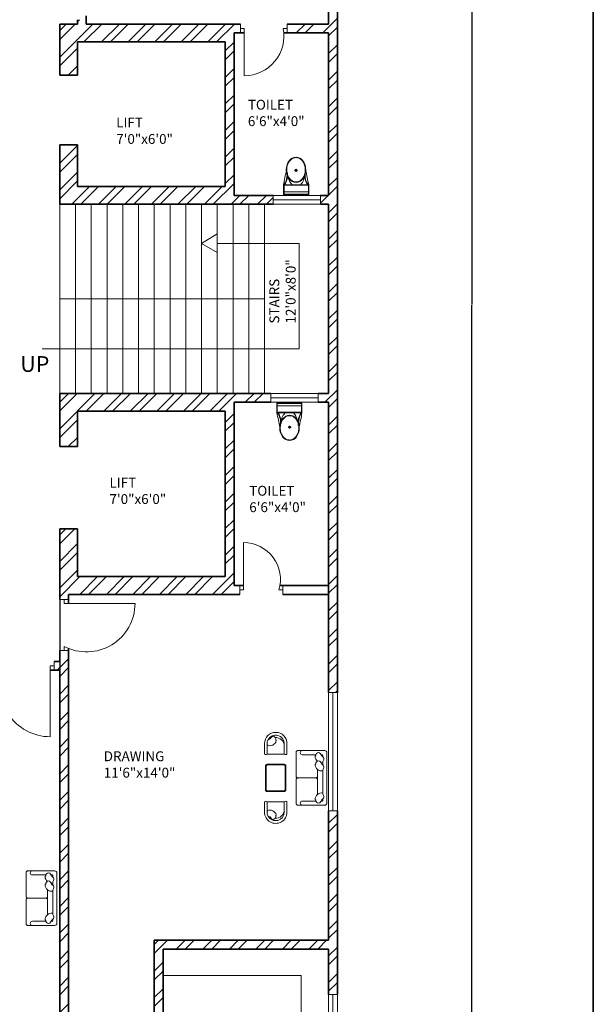
# Model space of a CAD drawing. Units: inches. Extents: x 1885 to 2748, y 783 to 2421.
# Tile 54 of 117: x 2457 to 2748, y 1350 to 1850. Entities that reach past the tile are written whole.
import ezdxf

# ---------------------------------------------------------------- set-up
doc = ezdxf.new("R2010")
doc.units = ezdxf.units.IN
for name, color, linetype, lineweight in [('A-ANNO-DIMS', 2, 'Continuous', 18), ('A-ANNO-SYMB', 81, 'Continuous', 18), ('A-ANNO-TTLB', 7, 'Continuous', 35), ('A-AREA-IDEN', 7, 'Continuous', 18), ('A-DOOR', 31, 'Continuous', 18), ('A-FLOR-CASE', 9, 'Continuous', 18), ('A-FLOR-FIXT', 8, 'Continuous', 18), ('A-FLOR-STRS', 81, 'Continuous', 18), ('A-FURN', 8, 'Continuous', 13), ('A-GLAZ', 181, 'Continuous', 18), ('A-WALL', 7, 'Continuous', 35)]:
    doc.layers.add(name, color=color, linetype=linetype, lineweight=lineweight)
doc.layers.add('A-WALL-PATT', color=85, linetype='Continuous', lineweight=13, true_color=0x58ba48)
doc.styles.get("Standard").update_dxf_attribs({"font": 'arial.ttf'})
doc.dimstyles.get("Standard").update_dxf_attribs({"dimtxt": 0.18, "dimasz": 0.18, "dimexe": 0.18, "dimexo": 0.0625, "dimgap": 0.09, "dimtad": 0, "dimtih": 1, "dimtoh": 1, "dimdec": 4, "dimzin": 0, "dimdsep": 46, "dimtxsty": 'Standard', "dimcen": 0.09, "dimadec": 0, "dimazin": 0, "dimtfac": 1, "dimtdec": 4, "dimtofl": 0, "dimtmove": 0, "dimatfit": 3, "dimfxl": 1, "dimtolj": 1, "dimtzin": 0, "dimarcsym": 0})

# ---------------------------------------------------------------- blocks, each defined once
blk = doc.blocks.new('A$C31115884')
for p, q in [((283, 498), (223, 498)), ((258, 466), (258, 523)), ((0, 200), (0, 0)), ((520, 200), (0, 200)), ((510, 54), (0, 54)), ((10, 190), (10, 10)), ((510, 190), (10, 190)), ((10, 10), (510, 10)), ((510, 10), (510, 190)), ((520, 0), (520, 200)), ((0, 0), (520, 0))]:
    blk.add_line(p, q)
blk.add_circle((256, 496), 23.6)
for centre, radius, start, end in [((2778, -205), 2807, 165.4549, 171.7133), ((-295, 403), 365, 324.2091, 9.3499), ((-295, 403), 375, 324.2091, 9.3499), ((139, 406), 293, 315.8436, 2.6563), ((806, 403), 375, 179.2036, 215.7909), ((806, 403), 365, 170.6501, 215.7909), ((3237, 905), 2807, 188.2867, 194.5451), ((384, 406), 293, 190.2774, 224.1564)]:
    blk.add_arc(centre, radius, start, end)
blk.add_ellipse((256, 510), major_axis=(0, -261), ratio=0.772727)
blk.add_open_spline([(256, 259), (263, 259), (270, 260), (288, 262), (299, 265), (320, 273), (330, 278), (350, 291), (360, 299), (378, 316), (386, 326), (402, 347), (409, 358), (421, 383), (427, 395), (436, 422), (440, 436), (445, 465), (447, 480), (448, 509), (448, 524), (445, 553), (443, 568), (436, 596), (432, 610), (422, 636), (416, 649), (402, 672), (395, 683), (379, 703), (370, 712), (351, 728), (341, 735), (321, 746), (310, 751), (289, 757), (278, 759), (256, 761), (245, 761), (223, 757), (212, 754), (191, 746), (181, 741), (161, 728), (151, 720), (133, 703), (125, 693), (110, 672), (103, 660), (90, 636), (85, 623), (76, 596), (72, 582), (67, 553), (66, 538), (64, 509), (65, 494), (68, 465), (70, 450), (77, 422), (81, 408), (91, 382), (97, 370), (111, 346), (118, 335), (135, 316), (144, 307), (162, 291), (172, 284), (193, 273), (203, 269), (225, 262), (236, 260), (250, 259), (253, 259), (256, 259)], degree=3, knots=[0, 0, 0, 0, 0.110105, 0.110105, 0.285049, 0.285049, 0.459994, 0.459994, 0.634938, 0.634938, 0.809882, 0.809882, 0.984827, 0.984827, 1.159771, 1.159771, 1.334715, 1.334715, 1.50966, 1.50966, 1.684604, 1.684604, 1.859549, 1.859549, 2.034493, 2.034493, 2.209437, 2.209437, 2.384382, 2.384382, 2.559326, 2.559326, 2.73427, 2.73427, 2.909215, 2.909215, 3.084159, 3.084159, 3.259103, 3.259103, 3.434048, 3.434048, 3.608992, 3.608992, 3.783936, 3.783936, 3.958881, 3.958881, 4.133825, 4.133825, 4.30877, 4.30877, 4.483714, 4.483714, 4.658658, 4.658658, 4.833603, 4.833603, 5.008547, 5.008547, 5.183491, 5.183491, 5.358436, 5.358436, 5.53338, 5.53338, 5.708324, 5.708324, 5.883269, 5.883269, 6.058213, 6.058213, 6.233158, 6.233158, 6.283185, 6.283185, 6.283185, 6.283185])
blk = doc.blocks.new('A$C1352')
at = {"color": 0}
for points in [[(0.003, 0.053), (0.003, 0.553, -0.414214), (0.053, 0.603), (0.753, 0.603, -0.414214), (0.803, 0.553), (0.803, 0.053, -0.414214), (0.753, 0.003), (0.053, 0.003, -0.414214)], [(0.023, 0.053), (0.023, 0.553, -0.414214), (0.053, 0.583), (0.753, 0.583, -0.414214), (0.783, 0.553), (0.783, 0.053, -0.414214), (0.753, 0.023), (0.053, 0.023, -0.414214)]]:
    blk.add_lwpolyline(points, format="xyb", close=True, dxfattribs=at)
blk = doc.blocks.new('CHAIR-LOUNGE')
blk.add_line((1.39, 5.7), (1.38, 10.98))
at = {"ltscale": 0.03}
blk.add_lwpolyline([(1.38, 10.98, 0.369229), (0, 10.98), (0, 5.7, 1), (11.42, 5.71), (11.42, 10.99, 0.369229), (10.03, 10.99)], format="xyb", close=True, dxfattribs=at)
blk.add_lwpolyline([(1.88, 3.71, 0.785087), (10.04, 5.71), (10.03, 10.99)], format="xyb")
for centre, radius, start, end in [((3.01, 5.02), 1.73, 145.8599, 267.0078), ((5.71, 5.71), 4.33, 180.0539, 181.1464), ((2.75, 3.42), 3.35, 15.7143, 112.9857), ((5.71, 6.93), 4.33, 266.342, 0.0539), ((4.77, 3.91), 1.95, 198.6466, 265.0001), ((3.98, 3.63), 1.78, 290.5305, 13.3597), ((5.79, 4.23), 0.207, 246.2577, 29.3762)]:
    blk.add_arc(centre, radius, start, end)
blk = doc.blocks.new('WIN-24')
for p, q in [((0, 4.5), (0, 0)), ((0, 4.5), (24, 4.5)), ((0, 0), (0, 2.25)), ((0, 2.25), (24, 2.25)), ((24, 2.25), (24, 4.5)), ((24, 4.5), (24, 0)), ((24, 0), (0, 0))]:
    blk.add_line(p, q)
blk = doc.blocks.new('WIN-36')
for p, q in [((0, 36), (4.5, 36)), ((0, 36), (0, 0)), ((4.5, 36), (2.25, 36)), ((2.25, 36), (2.25, 0)), ((4.5, 36), (4.5, 0)), ((2.25, 0), (0, 0)), ((0, 0), (4.5, 0))]:
    blk.add_line(p, q)
blk = doc.blocks.new('WIN-60-ALT')
for p, q in [((0, 60), (4.5, 60)), ((0, 60), (0, 0)), ((4.5, 60), (2.25, 60)), ((2.25, 60), (2.25, 0)), ((4.5, 0), (4.5, 60)), ((4.5, 0), (0, 0)), ((2.25, 0), (4.5, 0))]:
    blk.add_line(p, q)
blk = doc.blocks.new('*D44')
at = {"layer": 'A-ANNO-DIMS', "color": 0, "lineweight": -2, "transparency": 16777216}
for p, q in [((2618.34, 2352.51), (2686.7, 2352.51)), ((2686.52, 2352.33), (2686.52, 1705.19)), ((2686.52, 1057.69), (2686.52, 1704.82)), ((2618.34, 1057.51), (2686.7, 1057.51))]:
    blk.add_line(p, q, dxfattribs=at)
at = {"layer": 'A-ANNO-DIMS', "color": 0, "transparency": 16777216}
for points in [[(2686.49, 2352.33), (2686.55, 2352.33), (2686.52, 2352.51)], [(2686.49, 1057.69), (2686.55, 1057.69), (2686.52, 1057.51)]]:
    blk.add_solid(points, dxfattribs=at)
at = {"layer": 'Defpoints', "color": 0, "transparency": 16777216}
for p in [(2618.27, 2352.51), (2686.52, 2352.51), (2618.27, 1057.51)]:
    blk.add_point(p, dxfattribs=at)
at = {"layer": 'A-ANNO-DIMS', "color": 0, "transparency": 16777216, "insert": (2686.52, 1705.01), "char_height": 0.18, "attachment_point": 5}
blk.add_mtext('\\A1;1295', dxfattribs=at)
blk = doc.blocks.new('*D55')
at = {"layer": 'A-ANNO-DIMS', "color": 0, "lineweight": -2, "transparency": 16777216}
for p, q in [((2447.27, 1557.94), (2447.27, 922.48)), ((2477.27, 1557.94), (2477.27, 922.48)), ((2447.45, 922.66), (2462.06, 922.66)), ((2477.09, 922.66), (2462.49, 922.66))]:
    blk.add_line(p, q, dxfattribs=at)
at = {"layer": 'A-ANNO-DIMS', "color": 0, "transparency": 16777216}
for points in [[(2447.45, 922.69), (2447.45, 922.63), (2447.27, 922.66)], [(2477.09, 922.69), (2477.09, 922.63), (2477.27, 922.66)]]:
    blk.add_solid(points, dxfattribs=at)
at = {"layer": 'Defpoints', "color": 0, "transparency": 16777216}
for p in [(2447.27, 1558.01), (2477.27, 1558.01), (2477.27, 922.66)]:
    blk.add_point(p, dxfattribs=at)
at = {"layer": 'A-ANNO-DIMS', "color": 0, "transparency": 16777216, "insert": (2462.27, 922.66), "char_height": 0.18, "attachment_point": 5}
blk.add_mtext('\\A1;30', dxfattribs=at)

msp = doc.modelspace()

# ---------------------------------------------------------------- hatches: boundary and pattern name
at = {"layer": 'A-WALL-PATT'}
h = msp.add_hatch(dxfattribs=at)
h.set_pattern_fill('ANSI32', color=256)
h.paths.add_polyline_path([(2007.77, 2318.01), (1980.77, 2318.01), (1980.77, 2281.22), (1985.27, 2281.22), (1985.27, 2313.51), (2007.77, 2313.51), (2007.77, 2315.76)])
h.paths.add_polyline_path([(2094.32, 2318.01), (2067.77, 2318.01), (2067.77, 2313.51), (2094.32, 2313.51), (2094.32, 2315.76)])
h.paths.add_polyline_path([(2131.37, 2315.76), (2131.37, 2318.01), (2131.19, 2318.01), (2112.61, 2318.01), (2112.61, 2313.51), (2117.27, 2313.51), (2117.27, 2255.2), (2121.77, 2255.2), (2121.77, 2313.51), (2131.37, 2313.51)])
h.paths.add_polyline_path([(2190.51, 2318.01), (2155.37, 2318.01), (2155.37, 2313.51), (2169.77, 2313.51), (2169.77, 2229.51), (2121.77, 2229.51), (2121.77, 2233.45), (2119.52, 2233.45), (2117.27, 2233.45), (2117.27, 2201.1), (2121.77, 2201.1), (2121.77, 2225.01), (2169.77, 2225.01), (2169.77, 2165.01), (2306.27, 2165.01), (2306.27, 2066.01), (2310.77, 2066.01), (2344.27, 2066.01), (2486.27, 2066.01), (2486.27, 1886.01), (2483.02, 1886.01), (2483.02, 1881.51), (2486.27, 1881.51), (2486.27, 1880.68), (2490.77, 1880.68), (2490.77, 2070.51), (2344.27, 2070.51), (2310.77, 2070.51), (2310.77, 2165.01), (2310.77, 2173.64), (2308.52, 2173.64), (2306.27, 2173.64), (2306.27, 2169.51), (2174.27, 2169.51), (2174.27, 2313.51), (2190.51, 2313.51), (2190.51, 2315.76)])
h.paths.add_polyline_path([(1985.27, 2221.22), (1980.77, 2221.22), (1980.77, 2165.01), (1992.77, 2165.01), (1992.77, 2141.93), (1997.27, 2141.93), (1997.27, 2165.01), (2117.27, 2165.01), (2117.27, 2163.13), (2121.77, 2163.13), (2121.77, 2172.73), (2119.52, 2172.73), (2117.27, 2172.73), (2117.27, 2169.51), (1985.27, 2169.51)])
h.paths.add_polyline_path([(1997.27, 2105.93), (1992.77, 2105.93), (1992.77, 2070.51), (2016.77, 2070.51), (2016.77, 2059.12), (2019.02, 2059.12), (2021.27, 2059.12), (2021.27, 2070.51), (2117.27, 2070.51), (2117.27, 2022.51), (2114.42, 2022.51), (2114.42, 2018.01), (2123.63, 2018.01), (2123.63, 2020.26), (2123.63, 2022.51), (2121.77, 2022.51), (2121.77, 2142.59), (2119.52, 2142.59), (2117.27, 2142.59), (2117.27, 2075.01), (1997.27, 2075.01)])
h.paths.add_polyline_path([(2092.03, 2020.26), (2092.03, 2022.51), (2021.27, 2022.51), (2021.27, 2035.12), (2016.77, 2035.12), (2016.77, 2018.01), (2016.77, 1978.78), (2021.27, 1978.78), (2021.27, 2018.01), (2092.03, 2018.01)])
h.paths.add_polyline_path([(2260.94, 2022.51), (2153.1, 2022.51), (2153.1, 2020.26), (2153.1, 2018.01), (2155.27, 2018.01), (2155.27, 1886.01), (2107.63, 1886.01), (2107.63, 1881.51), (2182.91, 1881.51), (2182.91, 1883.76), (2182.91, 1886.01), (2159.77, 1886.01), (2159.77, 2018.01), (2260.94, 2018.01), (2260.94, 2020.26)])
h.paths.add_polyline_path([(2047.63, 1883.76), (2047.63, 1886.01), (2021.27, 1886.01), (2021.27, 1918.78), (2019.02, 1918.78), (2016.77, 1918.78), (2016.77, 1881.51), (2047.63, 1881.51)])
h.paths.add_polyline_path([(2306.36, 1883.76), (2306.36, 1886.01), (2296.27, 1886.01), (2296.27, 1982.01), (2316.54, 1982.01), (2316.54, 1984.26), (2316.54, 1986.51), (2296.27, 1986.51), (2296.27, 2022.51), (2289.28, 2022.51), (2289.28, 2018.01), (2291.77, 2018.01), (2291.77, 1886.01), (2242.91, 1886.01), (2242.91, 1881.51), (2306.36, 1881.51)], flags=17)
h.paths.add_polyline_path([(1985.27, 1843.01), (2021.6, 1843.01), (2021.53, 1845.44), (2021.48, 1847.51), (1980.77, 1847.51), (1980.77, 1809.45), (1985.27, 1809.45)])
h.paths.add_polyline_path([(2131.48, 1845.26), (2131.48, 1847.51), (2081.53, 1847.51), (2081.53, 1843.01), (2117.27, 1843.01), (2117.27, 1784.15), (2119.52, 1784.15), (2121.77, 1784.15), (2121.77, 1843.01), (2131.48, 1843.01)])
h.paths.add_polyline_path([(2203.89, 1847.51), (2155.48, 1847.51), (2155.48, 1843.01), (2169.77, 1843.01), (2169.77, 1759.01), (2121.77, 1759.01), (2121.77, 1761.46), (2117.27, 1761.46), (2117.27, 1730.43), (2121.77, 1730.43), (2121.77, 1754.51), (2177.42, 1754.51), (2177.42, 1756.76), (2177.42, 1759.01), (2174.27, 1759.01), (2174.27, 1843.01), (2203.89, 1843.01)])
h.paths.add_polyline_path([(2335.55, 1845.26), (2335.55, 1847.51), (2239.89, 1847.51), (2239.89, 1843.01), (2306.27, 1843.01), (2306.27, 1759.01), (2199.49, 1759.01), (2199.49, 1754.51), (2310.77, 1754.51), (2310.77, 1843.01), (2335.55, 1843.01)])
h.paths.add_polyline_path([(2348.77, 2022.51), (2344.27, 2022.51), (2344.27, 1986.51), (2341.68, 1986.51), (2341.68, 1982.01), (2344.27, 1982.01), (2344.27, 1886.01), (2330.36, 1886.01), (2330.36, 1881.51), (2361.63, 1881.51), (2361.63, 1883.76), (2361.63, 1886.01), (2348.77, 1886.01)], flags=17)
h.paths.add_polyline_path([(2283.25, 2315.76), (2283.25, 2318.01), (2238.51, 2318.01), (2238.51, 2313.51), (2283.25, 2313.51)], flags=17)
h.paths.add_polyline_path([(2363.27, 2348.01), (2388.68, 2348.01), (2388.68, 2350.26), (2388.68, 2352.51), (2358.77, 2352.51), (2358.77, 2348.01), (2358.77, 2318.01), (2344.48, 2318.01), (2344.48, 2313.51), (2358.77, 2313.51), (2358.77, 2229.51), (2310.77, 2229.51), (2310.77, 2231.95), (2306.27, 2231.95), (2306.27, 2205.61), (2310.77, 2205.61), (2310.77, 2225.01), (2358.77, 2225.01), (2358.77, 2211.51), (2452.33, 2211.51), (2452.33, 2213.76), (2452.33, 2216.01), (2363.27, 2216.01), (2363.27, 2318.01)])
h.paths.add_polyline_path([(2310.77, 2313.51), (2320.48, 2313.51), (2320.48, 2315.76), (2320.48, 2318.01), (2302.73, 2318.01), (2302.73, 2313.51), (2306.27, 2313.51), (2306.27, 2251.08), (2310.77, 2251.08)], flags=17)
h.paths.add_polyline_path([(2490.77, 2352.51), (2486.27, 2352.51), (2448.68, 2352.51), (2448.68, 2348.01), (2486.27, 2348.01), (2486.27, 2318.01), (2486.27, 2216.01), (2481.78, 2216.01), (2481.78, 2211.51), (2486.27, 2211.51), (2486.27, 2165.01), (2493.29, 2165.01), (2493.29, 2167.26), (2493.29, 2169.51), (2490.77, 2169.51), (2490.77, 2313.51), (2494.43, 2313.51), (2494.43, 2318.01), (2490.77, 2318.01)])
h.paths.add_polyline_path([(2534.65, 2318.01), (2515.69, 2318.01), (2515.69, 2313.51), (2534.65, 2313.51), (2534.65, 2315.76)])
h.paths.add_polyline_path([(2618.27, 2318.01), (2594.65, 2318.01), (2594.65, 2313.51), (2613.77, 2313.51), (2613.77, 2281.71), (2618.27, 2281.71)])
h.paths.add_polyline_path([(2618.27, 2221.71), (2613.77, 2221.71), (2613.77, 2169.51), (2554.02, 2169.51), (2554.02, 2165.01), (2613.77, 2165.01), (2613.77, 2152.88), (2618.27, 2152.88)])
h.paths.add_polyline_path([(2618.27, 2128.88), (2616.02, 2128.88), (2613.77, 2128.88), (2613.77, 2117.01), (2529.77, 2117.01), (2529.77, 2165.01), (2532.85, 2165.01), (2532.85, 2169.51), (2522.87, 2169.51), (2522.87, 2165.01), (2525.27, 2165.01), (2525.27, 2117.01), (2525.27, 2112.51), (2525.27, 2108.58), (2529.77, 2108.58), (2529.77, 2112.51), (2613.77, 2112.51), (2613.77, 2080.19), (2618.27, 2080.19)])
h.paths.add_polyline_path([(2618.27, 2044.19), (2616.02, 2044.19), (2613.77, 2044.19), (2613.77, 2015.51), (2529.77, 2015.51), (2529.77, 2088.58), (2527.52, 2088.58), (2525.27, 2088.58), (2525.27, 2011.01), (2613.77, 2011.01), (2613.77, 1956.75), (2618.27, 1956.75)])
h.paths.add_polyline_path([(2618.27, 1881.51), (2618.27, 1896.75), (2613.77, 1896.75), (2613.77, 1881.51), (2613.77, 1847.51), (2592.71, 1847.51), (2592.71, 1843.01), (2613.77, 1843.01), (2613.77, 1765.01), (2613.77, 1760.51), (2609.62, 1760.51), (2609.62, 1756.01), (2613.77, 1756.01), (2613.77, 1660.01), (2608.54, 1660.01), (2608.54, 1655.51), (2613.77, 1655.51), (2613.77, 1508.16), (2618.27, 1508.16)])
h.paths.add_polyline_path([(2565.77, 1843.01), (2569, 1843.01), (2569, 1847.51), (2490.77, 1847.51), (2490.77, 1849.7), (2488.52, 1849.7), (2486.27, 1849.7), (2486.27, 1847.51), (2477.27, 1847.51), (2477.27, 1838.51), (2477.27, 1821.49), (2486.27, 1821.49), (2486.27, 1838.51), (2561.27, 1838.51), (2561.27, 1765.01), (2486.27, 1765.01), (2486.27, 1786.16), (2477.27, 1786.16), (2477.27, 1765.01), (2477.27, 1756.01), (2486.27, 1756.01), (2565.77, 1756.01), (2585.62, 1756.01), (2585.62, 1758.26), (2585.62, 1760.51), (2565.77, 1760.51), (2565.77, 1765.01)])
h.paths.add_polyline_path([(2486.27, 1651.01), (2561.27, 1651.01), (2561.27, 1567.01), (2486.27, 1567.01), (2486.27, 1591.32), (2477.27, 1591.32), (2477.27, 1567.01), (2477.27, 1558.01), (2477.27, 1555.44), (2481.77, 1555.44), (2481.77, 1558.01), (2568.65, 1558.01), (2568.65, 1560.26), (2568.65, 1562.51), (2565.77, 1562.51), (2565.77, 1655.51), (2584.54, 1655.51), (2584.54, 1657.76), (2584.54, 1660.01), (2565.77, 1660.01), (2486.27, 1660.01), (2477.27, 1660.01), (2477.27, 1651.01), (2477.27, 1632.99), (2486.27, 1632.99)])
h.paths.add_polyline_path([(2449.97, 1883.76), (2449.97, 1886.01), (2421.63, 1886.01), (2421.63, 1881.51), (2449.97, 1881.51)], flags=17)
h.paths.add_polyline_path([(2447.27, 1847.51), (2395.55, 1847.51), (2395.55, 1843.01), (2442.77, 1843.01), (2442.77, 1809.27), (2447.27, 1809.27)])
h.paths.add_polyline_path([(1985.27, 1749.45), (1980.77, 1749.45), (1980.77, 1694.5), (1985.27, 1694.5), (1985.27, 1694.51), (1986.9, 1694.51), (1986.9, 1697.78), (1986.9, 1699.01), (1985.27, 1699.01)])
h.paths.add_polyline_path([(2152.77, 1699.01), (2121.77, 1699.01), (2121.77, 1703.67), (2119.52, 1703.67), (2117.27, 1703.67), (2117.27, 1699.01), (2009.22, 1699.01), (2009.22, 1694.51), (2148.27, 1694.51), (2148.27, 1692.63), (2152.77, 1692.63)])
h.paths.add_polyline_path([(2016.27, 1694.51), (2011.77, 1694.51), (2011.77, 1558.01), (2040.81, 1558.01), (2040.81, 1560.26), (2040.81, 1562.51), (2016.27, 1562.51)])
h.paths.add_polyline_path([(2152.77, 1663.02), (2150.52, 1663.02), (2148.27, 1663.02), (2148.27, 1562.51), (2100.81, 1562.51), (2100.81, 1558.01), (2165.12, 1558.01), (2165.12, 1560.26), (2165.12, 1562.51), (2152.77, 1562.51), (2152.77, 1610.51), (2224.77, 1610.51), (2224.77, 1607.99), (2229.27, 1607.99), (2229.27, 1615.01), (2152.77, 1615.01)])
h.paths.add_polyline_path([(2238.61, 1560.26), (2238.61, 1562.51), (2229.27, 1562.51), (2229.27, 1588.76), (2227.02, 1588.76), (2224.77, 1588.77), (2224.77, 1562.51), (2189.12, 1562.51), (2189.12, 1558.01), (2238.61, 1558.01)])
h.paths.add_polyline_path([(2336.02, 1560.26), (2336.02, 1562.51), (2310.77, 1562.51), (2310.77, 1656.35), (2308.52, 1656.35), (2306.27, 1656.35), (2306.27, 1562.51), (2286.61, 1562.51), (2286.61, 1558.01), (2336.02, 1558.01)])
h.paths.add_polyline_path([(2447.27, 1690.97), (2445.02, 1690.97), (2442.77, 1690.97), (2442.77, 1687.01), (2306.27, 1687.01), (2306.27, 1680.75), (2310.77, 1680.75), (2310.77, 1682.51), (2442.77, 1682.51), (2442.77, 1562.51), (2396.02, 1562.51), (2396.02, 1558.01), (2447.27, 1558.01)])
h.paths.add_polyline_path([(2447.27, 1749.27), (2445.02, 1749.27), (2442.77, 1749.27), (2442.77, 1717.23), (2447.27, 1717.23)])
h.paths.add_polyline_path([(2044.67, 1521.76), (2044.67, 1524.01), (2007.27, 1524.01), (2007.27, 1503.49), (2009.52, 1503.49), (2011.77, 1503.49), (2011.77, 1519.51), (2044.67, 1519.51)])
h.paths.add_polyline_path([(2177.97, 1521.76), (2177.97, 1524.01), (2104.67, 1524.01), (2104.67, 1519.51), (2145.77, 1519.51), (2145.77, 1387.51), (2143.37, 1387.51), (2143.37, 1383.01), (2251.59, 1383.01), (2251.59, 1385.26), (2251.59, 1387.51), (2150.27, 1387.51), (2150.27, 1519.51), (2177.97, 1519.51)])
h.paths.add_polyline_path([(2298.7, 1524.01), (2237.97, 1524.01), (2237.97, 1519.51), (2282.27, 1519.51), (2282.27, 1387.51), (2279.68, 1387.51), (2279.68, 1383.01), (2286.77, 1383.01), (2286.77, 1419.01), (2312.45, 1419.01), (2312.45, 1421.26), (2312.45, 1423.51), (2286.77, 1423.51), (2286.77, 1519.51), (2298.7, 1519.51), (2298.7, 1521.72)], flags=17)
h.paths.add_polyline_path([(2361.9, 1521.76), (2361.9, 1524.01), (2322.7, 1524.01), (2322.7, 1519.51), (2334.77, 1519.51), (2334.77, 1423.51), (2331.93, 1423.51), (2331.93, 1419.01), (2334.77, 1419.01), (2334.77, 1387.51), (2334.77, 1383.23), (2339.27, 1383.23), (2339.27, 1387.51), (2339.27, 1519.51), (2361.9, 1519.51)], flags=17)
h.paths.add_polyline_path([(2447.27, 1521.76), (2447.27, 1524.01), (2421.9, 1524.01), (2421.9, 1519.51), (2447.27, 1519.51)], flags=17)
h.paths.add_polyline_path([(2481.77, 1529.6), (2479.52, 1529.6), (2477.27, 1529.6), (2477.27, 1524.01), (2474.49, 1524.01), (2474.49, 1519.51), (2477.27, 1519.51), (2477.27, 1334.51), (2296.77, 1334.51), (2296.77, 1240.51), (2160.27, 1240.51), (2160.27, 1180.51), (2112.27, 1180.51), (2112.27, 1207.69), (2110.02, 1207.69), (2107.77, 1207.69), (2107.77, 1171.61), (2112.27, 1171.61), (2112.27, 1176.01), (2160.27, 1176.01), (2160.27, 1092.01), (2144.22, 1092.01), (2144.22, 1087.51), (2189.5, 1087.51), (2189.5, 1089.76), (2189.5, 1092.01), (2164.77, 1092.01), (2164.77, 1236.01), (2296.77, 1236.01), (2296.77, 1231.91), (2301.27, 1231.91), (2301.27, 1330.01), (2481.77, 1330.01), (2481.77, 1387.51)])
h.paths.add_polyline_path([(2618.27, 1448.16), (2613.77, 1448.16), (2613.77, 1382.51), (2529.77, 1382.51), (2525.27, 1382.51), (2525.27, 1307.06), (2529.77, 1307.06), (2529.77, 1378.01), (2613.77, 1378.01), (2613.77, 1354.99), (2618.27, 1354.99)])
h.paths.add_polyline_path([(2618.27, 1318.99), (2613.77, 1318.99), (2613.77, 1281.01), (2529.77, 1281.01), (2529.77, 1283.79), (2527.52, 1283.79), (2525.27, 1283.79), (2525.27, 1228.51), (2516.79, 1228.51), (2516.79, 1224.01), (2533.48, 1224.01), (2533.48, 1226.26), (2533.48, 1228.51), (2529.77, 1228.51), (2529.77, 1276.51), (2613.77, 1276.51), (2613.77, 1266.02), (2618.27, 1266.02)])
h.paths.add_polyline_path([(2618.27, 1134.96), (2613.77, 1134.96), (2613.77, 1092.01), (2594.54, 1092.01), (2594.54, 1087.51), (2618.27, 1087.51)])
h.paths.add_polyline_path([(2534.54, 1092.01), (2509.77, 1092.01), (2509.77, 1087.51), (2534.54, 1087.51), (2534.54, 1089.76)])
h.paths.add_polyline_path([(2481.27, 1224.01), (2484.12, 1224.01), (2484.12, 1226.26), (2484.12, 1228.51), (2476.77, 1228.51), (2476.77, 1198.51), (2471.61, 1198.51), (2471.61, 1194.01), (2476.77, 1194.01), (2476.77, 1062.01), (2436.89, 1062.01), (2436.89, 1057.51), (2476.77, 1057.51), (2481.27, 1057.51), (2481.27, 1062.01), (2481.27, 1087.51), (2485.35, 1087.51), (2485.35, 1089.76), (2485.35, 1092.01), (2481.27, 1092.01), (2481.27, 1117.51)])
h.paths.add_polyline_path([(2439.9, 1198.51), (2349.27, 1198.51), (2349.27, 1194.01), (2349.27, 1180.51), (2301.27, 1180.51), (2301.27, 1201.9), (2299.02, 1201.9), (2296.77, 1201.9), (2296.77, 1172.34), (2299.02, 1172.34), (2301.27, 1172.34), (2301.27, 1176.01), (2349.27, 1176.01), (2349.27, 1092.01), (2334.45, 1092.01), (2334.45, 1087.51), (2349.27, 1087.51), (2349.27, 1057.51), (2353.77, 1057.51), (2376.89, 1057.51), (2376.89, 1059.76), (2376.89, 1062.01), (2353.77, 1062.01), (2353.77, 1087.51), (2353.77, 1180.51), (2353.77, 1194.01), (2439.9, 1194.01), (2439.9, 1196.26)])
h.paths.add_polyline_path([(2270.6, 1089.76), (2270.6, 1092.01), (2249.5, 1092.01), (2249.5, 1087.51), (2270.6, 1087.51)], flags=17)
h.paths.add_polyline_path([(2310.45, 1092.01), (2301.27, 1092.01), (2301.27, 1153.29), (2296.77, 1153.29), (2296.77, 1092.01), (2293.79, 1092.01), (2293.79, 1087.51), (2310.45, 1087.51), (2310.45, 1089.76)], flags=17)
h.paths.add_polyline_path([(2112.27, 1150.33), (2110.02, 1150.33), (2107.77, 1150.33), (2107.77, 1092.01), (2104.47, 1092.01), (2104.47, 1087.51), (2120.22, 1087.51), (2120.22, 1089.76), (2120.22, 1092.01), (2112.27, 1092.01)])
h.paths.add_polyline_path([(2082.17, 1092.01), (2058.14, 1092.01), (2058.14, 1087.51), (2082.17, 1087.51), (2082.17, 1089.76)])
h.paths.add_polyline_path([(1975.77, 1145.64), (1971.27, 1145.64), (1971.27, 1087.51), (1980.77, 1087.51), (1998.14, 1087.51), (1998.14, 1089.76), (1998.14, 1092.01), (1985.27, 1092.01), (1975.77, 1092.01)])
h.paths.add_polyline_path([(2112.27, 1244.38), (2110.02, 1244.38), (2107.77, 1244.38), (2107.77, 1240.51), (1992.27, 1240.51), (1992.27, 1271.01), (1987.77, 1271.01), (1987.77, 1240.51), (1980.77, 1240.51), (1975.77, 1240.51), (1971.27, 1240.51), (1971.27, 1205.64), (1975.77, 1205.64), (1975.77, 1236.01), (2107.77, 1236.01), (2107.77, 1233.44), (2112.27, 1233.44), (2112.27, 1236.01)])
h.paths.add_polyline_path([(2112.27, 1383.01), (2114.78, 1383.01), (2114.78, 1385.26), (2114.78, 1387.51), (2102.48, 1387.51), (2102.48, 1383.01), (2107.77, 1383.01), (2107.77, 1335.01), (2011.77, 1335.01), (2011.77, 1349.94), (2007.27, 1349.94), (2007.27, 1335.01), (1987.77, 1335.01), (1987.77, 1330.51), (1987.77, 1307.01), (1992.27, 1307.01), (1992.27, 1330.51), (2007.27, 1330.51), (2107.77, 1330.51), (2107.77, 1264.71), (2112.27, 1264.71)])
h.paths.add_polyline_path([(2077.86, 1387.51), (2011.77, 1387.51), (2011.77, 1390.04), (2009.52, 1390.04), (2007.27, 1390.04), (2007.27, 1373.94), (2011.77, 1373.94), (2011.77, 1383.01), (2077.86, 1383.01)])
h.paths.add_polyline_path([(2011.77, 1443.49), (2007.27, 1443.49), (2007.27, 1410.25), (2011.77, 1410.25)])

# ---------------------------------------------------------------- linework, layer by layer
at = {"layer": 'A-ANNO-SYMB'}
for p, q in [((2549.27, 1736.07), (2557.27, 1740.95)), ((2557.27, 1740.95), (2557.27, 1731.6)), ((2557.27, 1731.6), (2549.27, 1736.07)), ((2598.93, 1736.07), (2557.27, 1736.07)), ((2598.93, 1682.64), (2598.93, 1736.07)), ((2468.39, 1682.64), (2598.93, 1682.64))]:
    msp.add_line(p, q, dxfattribs=at)
at = {"layer": 'A-ANNO-TTLB'}
msp.add_lwpolyline([(1885.16, 2409.17), (2748.2, 2409.17), (2748.2, 922.58), (1885.16, 922.58)], close=True, dxfattribs=at)
at = {"layer": 'A-DOOR'}
for p, q in [((2569, 1843.01), (2569, 1847.51)), ((2569, 1847.51), (2569, 1845.26)), ((2569, 1845.26), (2571, 1845.26)), ((2571, 1845.26), (2571, 1821.26)), ((2592.71, 1845.26), (2590.71, 1845.26)), ((2592.71, 1847.51), (2592.71, 1843.01)), ((2592.71, 1843.01), (2592.71, 1845.26)), ((2570.65, 1560.26), (2570.65, 1584.26)), ((2570.65, 1560.26), (2570.65, 1584.26)), ((2568.65, 1562.51), (2568.65, 1558.01)), ((2568.65, 1558.01), (2568.65, 1560.26)), ((2568.65, 1560.26), (2570.65, 1560.26)), ((2590.6, 1560.26), (2588.6, 1560.26)), ((2590.6, 1562.51), (2590.6, 1558.01)), ((2590.6, 1558.01), (2590.6, 1560.26)), ((2477.27, 1555.44), (2481.77, 1555.44)), ((2481.77, 1555.44), (2479.52, 1555.44)), ((2479.52, 1555.44), (2479.52, 1553.44)), ((2479.52, 1553.44), (2515.52, 1553.44)), ((2477.27, 1529.6), (2481.77, 1529.6)), ((2479.52, 1529.6), (2479.52, 1531.6)), ((2481.77, 1529.6), (2479.52, 1529.6)), ((2474.49, 1521.76), (2472.49, 1521.76)), ((2472.49, 1521.76), (2472.49, 1485.76)), ((2474.49, 1524.01), (2474.49, 1519.51)), ((2474.49, 1519.51), (2474.49, 1521.76))]:
    msp.add_line(p, q, dxfattribs=at)
for centre, radius, start, end in [((2571, 1841.36), 20.1, 270, 11.1884), ((2570.65, 1565.55), 18.71, 343.5739, 90), ((2490.9, 1553.44), 24.62, 242.4859, 0), ((2472.49, 1511.24), 25.49, 155.6331, 270)]:
    msp.add_arc(centre, radius, start, end, dxfattribs=at)
at = {"layer": 'A-FLOR-CASE'}
for p, q in [((2529.77, 1364.58), (2599.89, 1364.58)), ((2599.89, 1364.58), (2599.89, 1281.01))]:
    msp.add_line(p, q, dxfattribs=at)
at = {"layer": 'A-FLOR-STRS'}
for p, q in [((2477.27, 1756.01), (2477.27, 1660.01)), ((2485.27, 1756.01), (2485.27, 1660.01)), ((2493.27, 1756.01), (2493.27, 1660.01)), ((2501.27, 1756.01), (2501.27, 1660.01)), ((2509.27, 1756.01), (2509.27, 1660.01)), ((2517.27, 1756.01), (2517.27, 1660.01)), ((2525.27, 1756.01), (2525.27, 1660.01)), ((2533.27, 1756.01), (2533.27, 1660.01)), ((2541.27, 1756.01), (2541.27, 1660.01)), ((2549.27, 1756.01), (2549.27, 1660.01)), ((2557.27, 1756.01), (2557.27, 1660.01)), ((2565.27, 1756.01), (2565.27, 1660.01)), ((2573.27, 1756.01), (2573.27, 1660.01)), ((2581.27, 1756.01), (2581.27, 1660.01)), ((2477.27, 1708.01), (2581.27, 1708.01))]:
    msp.add_line(p, q, dxfattribs=at)
at = {"layer": 'A-FURN'}
for p, q in [((2607.38, 1476.63), (2600.45, 1476.63)), ((2610, 1476.63), (2610.48, 1476.63)), ((2610.83, 1476.29), (2610.83, 1475.65)), ((2610.83, 1471.5), (2610.83, 1473.15)), ((2610.83, 1472.13), (2610.83, 1471.5)), ((2610.83, 1456.58), (2610.83, 1469)), ((2600.45, 1453.1), (2607.38, 1453.1)), ((2610, 1453.1), (2610.48, 1453.1)), ((2610.83, 1453.45), (2610.83, 1454.08)), ((2470.29, 1415.59), (2463.36, 1415.59)), ((2472.91, 1415.59), (2473.39, 1415.59)), ((2473.74, 1415.24), (2473.74, 1414.6)), ((2473.74, 1410.45), (2473.74, 1412.11)), ((2473.74, 1411.09), (2473.74, 1410.45)), ((2473.74, 1395.54), (2473.74, 1407.95)), ((2463.36, 1392.06), (2470.29, 1392.06)), ((2472.91, 1392.06), (2473.39, 1392.06)), ((2473.74, 1392.4), (2473.74, 1393.04))]:
    msp.add_line(p, q, dxfattribs=at)
at = {"layer": 'A-FURN', "ltscale": 0.03}
for points in [[(2598.03, 1464.86, 0.414214), (2597.33, 1464.17), (2597.33, 1451.72, 0.414214), (2598.03, 1451.02), (2611.87, 1451.02, 0.414214), (2612.91, 1452.06), (2612.91, 1477.67, 0.414214), (2611.87, 1478.71), (2598.03, 1478.71, 0.414214), (2597.33, 1478.02), (2597.33, 1465.57, 0.414214), (2598.03, 1464.87)], [(2460.94, 1403.81, 0.414214), (2460.24, 1403.12), (2460.24, 1390.67, 0.414214), (2460.94, 1389.98), (2474.78, 1389.98, 0.414214), (2475.82, 1391.02), (2475.82, 1416.63, 0.414214), (2474.78, 1417.66), (2460.94, 1417.66, 0.414214), (2460.24, 1416.97), (2460.24, 1404.52, 0.414214), (2460.94, 1403.83)]]:
    msp.add_lwpolyline(points, format="xyb", dxfattribs=at)
at = {"layer": 'A-FURN'}
for points in [[(2608.15, 1469.14), (2608.15, 1465.73, -0.414214), (2607.28, 1464.87), (2598.2, 1464.87, -0.414214), (2597.33, 1465.73), (2597.33, 1477.84, -0.414214), (2598.2, 1478.71)], [(2608.15, 1457.03), (2608.15, 1464, 0.414214), (2607.28, 1464.87), (2598.2, 1464.87, 0.414214), (2597.33, 1464), (2597.33, 1451.89, 0.414214), (2598.2, 1451.02)], [(2471.06, 1408.09), (2471.06, 1404.69, -0.414214), (2470.19, 1403.82), (2461.11, 1403.82, -0.414214), (2460.24, 1404.69), (2460.24, 1416.8, -0.414214), (2461.11, 1417.66)], [(2471.06, 1395.99), (2471.06, 1402.96, 0.414214), (2470.19, 1403.82), (2461.11, 1403.82, 0.414214), (2460.24, 1402.96), (2460.24, 1390.84, 0.414214), (2461.11, 1389.98)]]:
    msp.add_lwpolyline(points, format="xyb", dxfattribs=at)
for points in [[(2608.15, 1469.14), (2608.15, 1456.44)], [(2471.06, 1408.09), (2471.06, 1395.4)]]:
    msp.add_lwpolyline(points, dxfattribs=at)
for centre, radius, start, end in [((2600.45, 1477.67), 1.04, 90, 180), ((2600.45, 1477.67), 1.04, 180, 270), ((2607.12, 1475.84), 0.207, 52.155, 195.2735), ((2610.27, 1475.88), 3.35, 181.6116, 229.376), ((2609.03, 1475.98), 1.78, 96.4279, 179.257), ((2608.19, 1475.9), 1.95, 4.5439, 70.8974), ((2609.63, 1474.4), 1.73, 311.7572, 72.9051), ((2610.48, 1476.29), 0.346, 0, 90), ((2610.48, 1476.29), 0.346, 0, 90), ((2607.12, 1471.69), 0.207, 52.155, 195.2735), ((2610.27, 1471.72), 3.35, 181.6116, 278.883), ((2609.03, 1471.83), 1.78, 96.4279, 179.257), ((2608.19, 1471.75), 1.95, 4.5439, 70.8974), ((2610.27, 1475.88), 3.35, 264.881, 278.883), ((2609.63, 1470.25), 1.73, 311.7572, 72.9051), ((2610.27, 1453.85), 3.35, 81.117, 178.3884), ((2609.63, 1455.33), 1.73, 287.0949, 48.2428), ((2600.45, 1452.06), 1.04, 90, 180), ((2600.45, 1452.06), 1.04, 180, 270), ((2607.12, 1453.89), 0.207, 164.7265, 307.845), ((2609.03, 1453.75), 1.78, 180.743, 263.5721), ((2608.19, 1453.83), 1.95, 289.1026, 355.4561), ((2610.48, 1453.45), 0.346, 270, 0), ((2463.36, 1416.63), 1.04, 90, 180), ((2463.36, 1416.63), 1.04, 180, 270), ((2470.03, 1414.79), 0.207, 52.155, 195.2735), ((2473.18, 1414.83), 3.35, 181.6116, 229.376), ((2471.94, 1414.93), 1.78, 96.4279, 179.257), ((2471.1, 1414.86), 1.95, 4.5439, 70.8974), ((2472.54, 1413.36), 1.73, 311.7572, 72.9051), ((2473.39, 1415.24), 0.346, 0, 90), ((2473.39, 1415.24), 0.346, 0, 90), ((2470.03, 1410.64), 0.207, 52.155, 195.2735), ((2473.18, 1410.68), 3.35, 181.6116, 278.883), ((2471.94, 1410.78), 1.78, 96.4279, 179.257), ((2471.1, 1410.7), 1.95, 4.5439, 70.8974), ((2473.18, 1414.83), 3.35, 264.881, 278.883), ((2472.54, 1409.2), 1.73, 311.7572, 72.9051), ((2473.18, 1392.81), 3.35, 81.117, 178.3884), ((2472.54, 1394.29), 1.73, 287.0949, 48.2428), ((2463.36, 1391.02), 1.04, 90, 180), ((2463.36, 1391.02), 1.04, 180, 270), ((2470.03, 1392.85), 0.207, 164.7265, 307.845), ((2471.94, 1392.71), 1.78, 180.743, 263.5721), ((2471.1, 1392.78), 1.95, 289.1026, 355.4561), ((2473.39, 1392.4), 0.346, 270, 0)]:
    msp.add_arc(centre, radius, start, end, dxfattribs=at)
at = {"layer": 'A-WALL'}
for p, q in [((2613.77, 1847.51), (2613.77, 1881.51)), ((2618.27, 1881.51), (2618.27, 1508.16)), ((2486.27, 1849.7), (2486.27, 1847.51)), ((2490.77, 1851.7), (2490.77, 1847.51)), ((2477.27, 1847.51), (2486.27, 1847.51)), ((2477.27, 1838.51), (2477.27, 1847.51)), ((2477.27, 1847.51), (2486.27, 1847.51)), ((2490.77, 1847.51), (2569, 1847.51)), ((2592.71, 1847.51), (2613.77, 1847.51)), ((2565.77, 1843.01), (2565.77, 1765.01)), ((2571, 1843.01), (2565.77, 1843.01)), ((2613.77, 1843.01), (2591.03, 1843.01)), ((2613.77, 1765.01), (2613.77, 1843.01)), ((2477.27, 1838.51), (2477.27, 1821.49)), ((2561.27, 1838.51), (2486.27, 1838.51)), ((2486.27, 1838.51), (2486.27, 1821.49)), ((2561.27, 1765.01), (2561.27, 1838.51)), ((2477.27, 1821.49), (2486.27, 1821.49)), ((2486.27, 1786.16), (2477.27, 1786.16)), ((2477.27, 1786.16), (2477.27, 1765.01)), ((2486.27, 1786.16), (2486.27, 1765.01)), ((2477.27, 1756.01), (2477.27, 1765.01)), ((2486.27, 1765.01), (2561.27, 1765.01)), ((2565.77, 1765.01), (2565.77, 1760.51)), ((2613.77, 1765.01), (2613.77, 1760.51)), ((2565.77, 1760.51), (2585.62, 1760.51)), ((2609.62, 1760.51), (2613.77, 1760.51)), ((2486.27, 1756.01), (2477.27, 1756.01)), ((2486.27, 1756.01), (2565.77, 1756.01)), ((2565.77, 1756.01), (2585.62, 1756.01)), ((2609.62, 1756.01), (2613.77, 1756.01)), ((2613.77, 1660.01), (2613.77, 1756.01)), ((2477.27, 1651.01), (2477.27, 1660.01)), ((2477.27, 1660.01), (2486.27, 1660.01)), ((2486.27, 1660.01), (2565.77, 1660.01)), ((2565.77, 1660.01), (2584.54, 1660.01)), ((2608.54, 1660.01), (2613.77, 1660.01)), ((2565.77, 1655.51), (2584.54, 1655.51)), ((2565.77, 1562.51), (2565.77, 1655.51)), ((2608.54, 1655.51), (2613.77, 1655.51)), ((2613.77, 1508.16), (2613.77, 1655.51)), ((2477.27, 1651.01), (2477.27, 1632.99)), ((2561.27, 1651.01), (2486.27, 1651.01)), ((2486.27, 1632.99), (2486.27, 1651.01)), ((2561.27, 1651.01), (2561.27, 1567.01)), ((2477.27, 1632.99), (2486.27, 1632.99)), ((2477.27, 1591.32), (2486.27, 1591.32)), ((2477.27, 1591.32), (2477.27, 1567.01)), ((2486.27, 1567.01), (2486.27, 1591.32)), ((2477.27, 1567.01), (2477.27, 1558.01)), ((2561.27, 1567.01), (2486.27, 1567.01)), ((2570.65, 1562.51), (2565.77, 1562.51)), ((2613.77, 1562.51), (2589.11, 1562.51)), ((2613.77, 1558.01), (2613.77, 1562.51)), ((2477.27, 1558.01), (2477.27, 1555.44)), ((2481.77, 1558.01), (2568.65, 1558.01)), ((2481.77, 1558.01), (2481.77, 1553.44)), ((2590.6, 1558.01), (2613.77, 1558.01)), ((2477.27, 1529.6), (2477.27, 1524.01)), ((2481.77, 1530.57), (2481.77, 1387.51)), ((2472.49, 1519.51), (2477.27, 1519.51)), ((2474.49, 1524.01), (2477.27, 1524.01)), ((2477.27, 1519.51), (2477.27, 1387.51)), ((2477.27, 1519.51), (2477.27, 1334.51)), ((2613.77, 1382.51), (2613.77, 1448.16)), ((2618.27, 1448.16), (2618.27, 1354.99)), ((2481.77, 1330.01), (2481.77, 1387.51)), ((2525.27, 1382.51), (2613.77, 1382.51)), ((2525.27, 1307.06), (2525.27, 1382.51)), ((2613.77, 1382.51), (2529.77, 1382.51)), ((2529.77, 1378.01), (2613.77, 1378.01)), ((2529.77, 1378.01), (2529.77, 1305.42)), ((2613.77, 1354.99), (2613.77, 1378.01))]:
    msp.add_line(p, q, dxfattribs=at)

# ---------------------------------------------------------------- block references
at = {"layer": 'A-FLOR-FIXT', "xscale": 0.0246256636748975, "yscale": 0.0246256636748975, "zscale": 0.0246256636748975}
msp.add_blockref('A$C31115884', (2590.95, 1760.96), dxfattribs=at)
at = {"layer": 'A-FLOR-FIXT', "xscale": 0.0246256636748975, "yscale": 0.0246256636748975, "zscale": 0.0246256636748975, "rotation": 180}
msp.add_blockref('A$C31115884', (2600.26, 1655.09), dxfattribs=at)
at = {"layer": 'A-FURN', "extrusion": (0, 0, -1), "zscale": -1, "rotation": 180}
msp.add_blockref('CHAIR-LOUNGE', (-2581.24, 1487.96), dxfattribs=at)
at = {"layer": 'A-FURN', "ltscale": 0.03, "xscale": 17.30251319894821, "yscale": 17.30251319894821, "zscale": 17.30251319894821, "rotation": 270}
msp.add_blockref('A$C1352', (2581.71, 1471.83), dxfattribs=at)
at = {"layer": 'A-FURN'}
msp.add_blockref('CHAIR-LOUNGE', (2581.24, 1441.77), dxfattribs=at)
at = {"layer": 'A-GLAZ'}
for name, p in [('WIN-24', (2585.62, 1756.01)), ('WIN-24', (2584.54, 1655.51)), ('WIN-60-ALT', (2613.77, 1448.16)), ('WIN-36', (2613.77, 1318.99))]:
    msp.add_blockref(name, p, dxfattribs=at)

# ---------------------------------------------------------------- texts
at = {"layer": 'A-ANNO-SYMB', "insert": (2457.22, 1678.93), "char_height": 8, "attachment_point": 1}
msp.add_mtext_dynamic_manual_height_columns('UP ', width=36.0567, gutter_width=12.5, heights=[0], dxfattribs=at)
at = {"layer": 'A-AREA-IDEN', "char_height": 5, "attachment_point": 1}
for s, width, insert in [('TOILET\\P6\'6"x4\'0"', 95.8297, (2572.8, 1809.04)), ('LIFT\\P7\'0"x6\'0"', 76.0604, (2505.95, 1799.99)), ('LIFT\\P7\'0"x6\'0"', 160.1523, (2502.53, 1617.22)), ('TOILET\\P6\'6"x4\'0"', 209.6317, (2573.5, 1613.1)), ('DRAWING\\P11\'6"x14\'0"', 219.5353, (2499.63, 1478.35))]:
    msp.add_mtext_dynamic_manual_height_columns(s, width=width, gutter_width=12.5, heights=[0], dxfattribs=dict(at, insert=insert))
at = {"layer": 'A-AREA-IDEN', "insert": (2583.73, 1695.49), "char_height": 5, "attachment_point": 1, "rotation": 90}
msp.add_mtext_dynamic_manual_height_columns('STAIRS\\P12\'0"x8\'0"', width=105.8799, gutter_width=12.5, heights=[0], dxfattribs=at)

# ---------------------------------------------------------------- dimensions: what is measured, and where the dimension line sits
at = {"layer": 'A-ANNO-DIMS'}
dim = msp.add_linear_dim(base=(2686.52, 2352.51), p1=(2618.27, 1057.51), p2=(2618.27, 2352.51), angle=90, dimstyle='Standard', override={"dimdec": 0, "dimlfac": 1, "dimrnd": 0, "dimzin": 0, "dimdsep": 46, "dimlunit": 2}, dxfattribs=at)
dim.commit()
dim.dimension.update_dxf_attribs({"geometry": '*D44', "text_midpoint": (2686.52, 1705.01)})
dim = msp.add_linear_dim(base=(2477.27, 922.66), p1=(2447.27, 1558.01), p2=(2477.27, 1558.01), dimstyle='Standard', override={"dimdec": 0, "dimlfac": 1, "dimrnd": 0, "dimzin": 0, "dimdsep": 46, "dimlunit": 2}, dxfattribs=at)
dim.commit()
dim.dimension.update_dxf_attribs({"geometry": '*D55', "text_midpoint": (2462.27, 922.66)})

doc.saveas('drawing.dxf')
